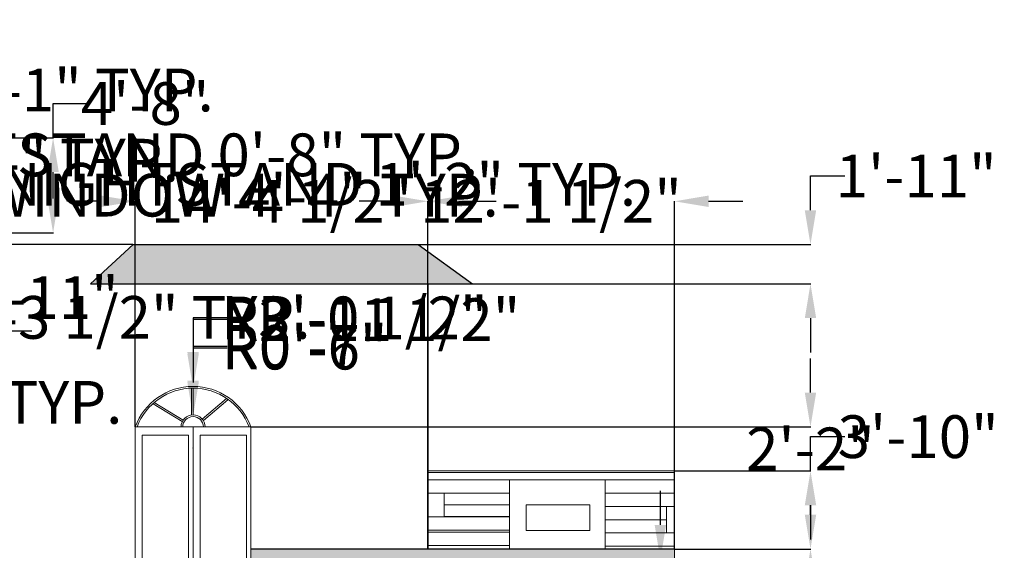
# Model space of a CAD drawing. Units: inches. Extents: x 28 to 3832, y 2 to 1709.
# Tile 6 of 7: x 2956 to 3536, y 1338 to 1651. Entities that reach past the tile are written whole.
import ezdxf

# ---------------------------------------------------------------- set-up
doc = ezdxf.new("R2010")
doc.units = ezdxf.units.IN
doc.header["$MEASUREMENT"] = 0
for name, color, linetype, lineweight in [('A-ANNO-DIMS', 2, 'Continuous', 18), ('A-ELEV', 7, 'Continuous', 30), ('A-ELEV-DETL', 7, 'Continuous', 18), ('A-ELEV-OPEN', 4, 'Continuous', 18), ('A-ELEV-ROOF', 7, 'Continuous', 25)]:
    doc.layers.add(name, color=color, linetype=linetype, lineweight=lineweight)
doc.layers.add('A-ELEV-PATT', color=252, linetype='Continuous', lineweight=9, true_color=0x939598)
doc.layers.add('A-ROOF-PATT', color=30, linetype='Continuous', lineweight=9, true_color=0xf8991e)
doc.styles.get("Standard").update_dxf_attribs({"font": 'arial.ttf'})
doc.dimstyles.get("Standard").update_dxf_attribs({"dimtxt": 25.18, "dimasz": 20.18, "dimexe": 0.18, "dimexo": 0.0625, "dimgap": 0.09, "dimtad": 0, "dimtih": 1, "dimtoh": 1, "dimdec": 0, "dimzin": 0, "dimdsep": 46, "dimlunit": 3, "dimtxsty": 'Standard', "dimcen": 0.09, "dimadec": 0, "dimazin": 0, "dimtfac": 1, "dimtdec": 0, "dimtofl": 0, "dimtmove": 0, "dimatfit": 3, "dimfxl": 1, "dimtolj": 1, "dimtzin": 0, "dimarcsym": 0})

# ---------------------------------------------------------------- blocks, each defined once
blk = doc.blocks.new('*D23')
at = {"layer": 'A-ANNO-DIMS', "color": 0, "lineweight": -2, "transparency": 16777216}
for p, q in [((2540.14, 1405.47), (2540.14, 1425.65)), ((2540.14, 1425.65), (2560.32, 1425.65)), ((2548.79, 1405.47), (2539.96, 1405.47)), ((2540.14, 1367.62), (2540.14, 1385.29)), ((2548.79, 1347.44), (2539.96, 1347.44))]:
    blk.add_line(p, q, dxfattribs=at)
at = {"layer": 'A-ANNO-DIMS', "color": 0, "transparency": 16777216}
for points in [[(2536.78, 1385.29), (2543.51, 1385.29), (2540.14, 1405.47)], [(2536.78, 1367.62), (2543.51, 1367.62), (2540.14, 1347.44)]]:
    blk.add_solid(points, dxfattribs=at)
at = {"layer": 'Defpoints', "color": 0, "transparency": 16777216}
for p in [(2540.14, 1405.47), (2548.85, 1405.47), (2548.85, 1347.44)]:
    blk.add_point(p, dxfattribs=at)
at = {"layer": 'A-ANNO-DIMS', "color": 0, "transparency": 16777216, "insert": (2795, 1425.65), "char_height": 25.18, "attachment_point": 5}
blk.add_mtext('\\A1;WINDOW SHADE 4\'-10" TYP.', dxfattribs=at)
blk = doc.blocks.new('*D25')
at = {"layer": 'A-ANNO-DIMS', "color": 0, "lineweight": -2, "transparency": 16777216}
for p, q in [((2905.84, 1527.52), (2905.84, 1547.7)), ((2905.84, 1547.7), (2926.02, 1547.7)), ((2913.58, 1527.52), (2905.66, 1527.52)), ((2905.84, 1495.7), (2905.84, 1507.34)), ((2913.58, 1475.52), (2905.66, 1475.52))]:
    blk.add_line(p, q, dxfattribs=at)
at = {"layer": 'A-ANNO-DIMS', "color": 0, "transparency": 16777216}
for points in [[(2902.48, 1507.34), (2909.2, 1507.34), (2905.84, 1527.52)], [(2902.48, 1495.7), (2909.2, 1495.7), (2905.84, 1475.52)]]:
    blk.add_solid(points, dxfattribs=at)
at = {"layer": 'Defpoints', "color": 0, "transparency": 16777216}
for p in [(2905.84, 1527.52), (2913.64, 1527.52), (2913.64, 1475.52)]:
    blk.add_point(p, dxfattribs=at)
at = {"layer": 'A-ANNO-DIMS', "color": 0, "transparency": 16777216, "insert": (3085.42, 1547.7), "char_height": 25.18, "attachment_point": 5}
blk.add_mtext('\\A1;WINDOW 4\'-4" TYP.', dxfattribs=at)
blk = doc.blocks.new('*D26')
at = {"layer": 'A-ANNO-DIMS', "color": 0, "lineweight": -2, "transparency": 16777216}
for p, q in [((2913.64, 1475.46), (2913.64, 1467.54)), ((2922.64, 1475.46), (2922.64, 1467.54)), ((2893.46, 1467.72), (2873.28, 1467.72)), ((2942.82, 1467.72), (2963, 1467.72))]:
    blk.add_line(p, q, dxfattribs=at)
at = {"layer": 'A-ANNO-DIMS', "color": 0, "transparency": 16777216}
for points in [[(2893.46, 1471.09), (2893.46, 1464.36), (2913.64, 1467.72)], [(2942.82, 1471.09), (2942.82, 1464.36), (2922.64, 1467.72)]]:
    blk.add_solid(points, dxfattribs=at)
at = {"layer": 'Defpoints', "color": 0, "transparency": 16777216}
for p in [(2913.64, 1475.52), (2922.64, 1475.52), (2913.64, 1467.72)]:
    blk.add_point(p, dxfattribs=at)
at = {"layer": 'A-ANNO-DIMS', "color": 0, "transparency": 16777216, "insert": (2796.45, 1467.72), "char_height": 25.18, "attachment_point": 5}
blk.add_mtext('\\A1;0\'-9" TYP.', dxfattribs=at)
blk = doc.blocks.new('*D31')
at = {"layer": 'A-ANNO-DIMS', "color": 0, "lineweight": -2, "transparency": 16777216}
for p, q in [((2653.18, 1475.69), (2633, 1475.69)), ((2673.36, 1469.86), (2673.36, 1475.87)), ((2712.64, 1469.86), (2712.64, 1475.87)), ((2732.82, 1475.69), (2753, 1475.69))]:
    blk.add_line(p, q, dxfattribs=at)
at = {"layer": 'A-ANNO-DIMS', "color": 0, "transparency": 16777216}
for points in [[(2653.18, 1479.05), (2653.18, 1472.33), (2673.36, 1475.69)], [(2732.82, 1479.05), (2732.82, 1472.33), (2712.64, 1475.69)]]:
    blk.add_solid(points, dxfattribs=at)
at = {"layer": 'Defpoints', "color": 0, "transparency": 16777216}
for p in [(2712.64, 1475.69), (2673.36, 1469.8), (2712.64, 1469.8)]:
    blk.add_point(p, dxfattribs=at)
at = {"layer": 'A-ANNO-DIMS', "color": 0, "transparency": 16777216, "insert": (2943.56, 1475.69), "char_height": 25.18, "attachment_point": 5}
blk.add_mtext('\\A1;DOOR D1 3\'-3 1/2" TYP.', dxfattribs=at)
blk = doc.blocks.new('*D35')
at = {"layer": 'A-ANNO-DIMS', "color": 0, "lineweight": -2, "transparency": 16777216}
for p, q in [((2708.46, 1568.32), (2688.28, 1568.32)), ((2728.64, 1572.46), (2728.64, 1568.14)), ((2756.64, 1572.46), (2756.64, 1568.14)), ((2776.82, 1568.32), (2797, 1568.32))]:
    blk.add_line(p, q, dxfattribs=at)
at = {"layer": 'A-ANNO-DIMS', "color": 0, "transparency": 16777216}
for points in [[(2708.46, 1571.69), (2708.46, 1564.96), (2728.64, 1568.32)], [(2776.82, 1571.69), (2776.82, 1564.96), (2756.64, 1568.32)]]:
    blk.add_solid(points, dxfattribs=at)
at = {"layer": 'Defpoints', "color": 0, "transparency": 16777216}
for p in [(2728.64, 1572.52), (2756.64, 1572.52), (2756.64, 1568.32)]:
    blk.add_point(p, dxfattribs=at)
at = {"layer": 'A-ANNO-DIMS', "color": 0, "transparency": 16777216, "insert": (2926.28, 1568.32), "char_height": 25.18, "attachment_point": 5}
blk.add_mtext('\\A1;VENT 2\'-4" TYP.', dxfattribs=at)
blk = doc.blocks.new('*D39')
at = {"layer": 'A-ANNO-DIMS', "color": 0, "lineweight": -2, "transparency": 16777216}
for p, q in [((2653.75, 1571.46), (2633.57, 1571.46)), ((2673.93, 1570.3), (2673.93, 1571.64)), ((2682.13, 1570.3), (2682.13, 1571.64)), ((2702.31, 1571.46), (2722.49, 1571.46))]:
    blk.add_line(p, q, dxfattribs=at)
at = {"layer": 'A-ANNO-DIMS', "color": 0, "transparency": 16777216}
for points in [[(2653.75, 1574.83), (2653.75, 1568.1), (2673.93, 1571.46)], [(2702.31, 1574.83), (2702.31, 1568.1), (2682.13, 1571.46)]]:
    blk.add_solid(points, dxfattribs=at)
at = {"layer": 'Defpoints', "color": 0, "transparency": 16777216}
for p in [(2673.93, 1570.23), (2682.13, 1571.46), (2682.13, 1570.23)]:
    blk.add_point(p, dxfattribs=at)
at = {"layer": 'A-ANNO-DIMS', "color": 0, "transparency": 16777216, "insert": (2981.04, 1571.46), "char_height": 25.18, "attachment_point": 5}
blk.add_mtext('\\A1;SMALL NIGHTSTAND 0\'-8" TYP.', dxfattribs=at)
blk = doc.blocks.new('*D41')
at = {"layer": 'A-ANNO-DIMS', "color": 0, "lineweight": -2, "transparency": 16777216}
for p, q in [((2881.52, 1556.14), (2881.52, 1553.93)), ((2895.49, 1556.14), (2895.49, 1553.93)), ((2861.34, 1554.11), (2841.16, 1554.11)), ((2915.67, 1554.11), (2935.85, 1554.11))]:
    blk.add_line(p, q, dxfattribs=at)
at = {"layer": 'A-ANNO-DIMS', "color": 0, "transparency": 16777216}
for points in [[(2861.34, 1557.47), (2861.34, 1550.74), (2881.52, 1554.11)], [(2915.67, 1557.47), (2915.67, 1550.74), (2895.49, 1554.11)]]:
    blk.add_solid(points, dxfattribs=at)
at = {"layer": 'Defpoints', "color": 0, "transparency": 16777216}
for p in [(2881.52, 1556.2), (2895.49, 1556.2), (2895.49, 1554.11)]:
    blk.add_point(p, dxfattribs=at)
at = {"layer": 'A-ANNO-DIMS', "color": 0, "transparency": 16777216, "insert": (3131.28, 1554.11), "char_height": 25.18, "attachment_point": 5}
blk.add_mtext('\\A1;NIGHTSTAND 1\'-2" TYP.', dxfattribs=at)
blk = doc.blocks.new('*D42')
at = {"layer": 'A-ANNO-DIMS', "color": 0, "lineweight": -2, "transparency": 16777216}
for p, q in [((2897.58, 1589.46), (2897.58, 1609.64)), ((2897.58, 1609.64), (2917.76, 1609.64)), ((2895.55, 1569.28), (2897.76, 1569.28)), ((2895.55, 1556.2), (2897.76, 1556.2)), ((2897.58, 1536.02), (2897.58, 1515.84))]:
    blk.add_line(p, q, dxfattribs=at)
at = {"layer": 'A-ANNO-DIMS', "color": 0, "transparency": 16777216}
for points in [[(2894.22, 1589.46), (2900.95, 1589.46), (2897.58, 1569.28)], [(2894.22, 1536.02), (2900.95, 1536.02), (2897.58, 1556.2)]]:
    blk.add_solid(points, dxfattribs=at)
at = {"layer": 'Defpoints', "color": 0, "transparency": 16777216}
for p in [(2895.49, 1569.28), (2897.58, 1569.28), (2895.49, 1556.2)]:
    blk.add_point(p, dxfattribs=at)
at = {"layer": 'A-ANNO-DIMS', "color": 0, "transparency": 16777216, "insert": (2993.41, 1609.64), "char_height": 25.18, "attachment_point": 5}
blk.add_mtext('\\A1;1\'-1" TYP.', dxfattribs=at)
blk = doc.blocks.new('*D45')
at = {"layer": 'A-ANNO-DIMS', "color": 0, "lineweight": -2, "transparency": 16777216}
for p, q in [((3166.51, 1302.58), (3166.51, 1280.67)), ((3311.78, 1302.58), (3311.78, 1280.67)), ((3186.69, 1280.85), (3291.6, 1280.85)), ((3311.78, 1280.85), (3331.96, 1280.85))]:
    blk.add_line(p, q, dxfattribs=at)
at = {"layer": 'A-ANNO-DIMS', "color": 0, "transparency": 16777216}
for points in [[(3186.69, 1284.21), (3186.69, 1277.49), (3166.51, 1280.85)], [(3291.6, 1284.21), (3291.6, 1277.49), (3311.78, 1280.85)]]:
    blk.add_solid(points, dxfattribs=at)
at = {"layer": 'Defpoints', "color": 0, "transparency": 16777216}
for p in [(3166.51, 1302.64), (3311.78, 1302.64), (3311.78, 1280.85)]:
    blk.add_point(p, dxfattribs=at)
at = {"layer": 'A-ANNO-DIMS', "color": 0, "transparency": 16777216, "insert": (3590.91, 1280.85), "char_height": 25.18, "attachment_point": 5}
blk.add_mtext('\\A1;ENTRY CANOPY 12\'-1 1/2" TYP.', dxfattribs=at)
blk = doc.blocks.new('*D46')
at = {"layer": 'A-ANNO-DIMS', "color": 0, "lineweight": -2, "transparency": 16777216}
for p, q in [((3333.57, 1353.41), (3333.57, 1373.59)), ((3311.84, 1333.23), (3333.75, 1333.23)), ((3311.84, 1302.64), (3333.75, 1302.64)), ((3333.57, 1282.46), (3333.57, 1262.28))]:
    blk.add_line(p, q, dxfattribs=at)
at = {"layer": 'A-ANNO-DIMS', "color": 0, "transparency": 16777216}
for points in [[(3330.21, 1353.41), (3336.94, 1353.41), (3333.57, 1333.23)], [(3330.21, 1282.46), (3336.94, 1282.46), (3333.57, 1302.64)]]:
    blk.add_solid(points, dxfattribs=at)
at = {"layer": 'Defpoints', "color": 0, "transparency": 16777216}
for p in [(3311.78, 1333.23), (3333.57, 1333.23), (3311.78, 1302.64)]:
    blk.add_point(p, dxfattribs=at)
at = {"layer": 'A-ANNO-DIMS', "color": 0, "transparency": 16777216, "insert": (3333.57, 1317.94), "char_height": 25.18, "attachment_point": 5}
blk.add_mtext('\\A1;2\'-6 1/2" TYP.', dxfattribs=at)
blk = doc.blocks.new('*D51')
at = {"layer": 'A-ANNO-DIMS', "color": 0, "lineweight": -2, "transparency": 16777216}
for p, q in [((2975.53, 1581.52), (2975.53, 1601.7)), ((2975.53, 1601.7), (2995.71, 1601.7)), ((2922.7, 1581.52), (2975.71, 1581.52)), ((2975.53, 1545.7), (2975.53, 1561.34)), ((2922.7, 1525.52), (2975.71, 1525.52))]:
    blk.add_line(p, q, dxfattribs=at)
at = {"layer": 'A-ANNO-DIMS', "color": 0, "transparency": 16777216}
for points in [[(2972.16, 1561.34), (2978.89, 1561.34), (2975.53, 1581.52)], [(2972.16, 1545.7), (2978.89, 1545.7), (2975.53, 1525.52)]]:
    blk.add_solid(points, dxfattribs=at)
at = {"layer": 'Defpoints', "color": 0, "transparency": 16777216}
for p in [(2922.64, 1581.52), (2975.53, 1581.52), (2922.64, 1525.52)]:
    blk.add_point(p, dxfattribs=at)
at = {"layer": 'A-ANNO-DIMS', "color": 0, "transparency": 16777216, "insert": (3029.77, 1601.7), "char_height": 25.18, "attachment_point": 5}
blk.add_mtext('\\A1;4\'-8"', dxfattribs=at)
blk = doc.blocks.new('*D54')
at = {"layer": 'A-ANNO-DIMS', "color": 0, "lineweight": -2, "transparency": 16777216}
for p, q in [((3022.59, 1518.63), (2935.04, 1518.63)), ((2935.22, 1498.45), (2935.22, 1303.17)), ((2935.22, 1081.98), (2935.22, 1277.26)), ((2960.61, 1061.8), (2935.04, 1061.8))]:
    blk.add_line(p, q, dxfattribs=at)
at = {"layer": 'A-ANNO-DIMS', "color": 0, "transparency": 16777216}
for points in [[(2931.86, 1498.45), (2938.58, 1498.45), (2935.22, 1518.63)], [(2931.86, 1081.98), (2938.58, 1081.98), (2935.22, 1061.8)]]:
    blk.add_solid(points, dxfattribs=at)
at = {"layer": 'Defpoints', "color": 0, "transparency": 16777216}
for p in [(2935.22, 1518.63), (3022.65, 1518.63), (2960.67, 1061.8)]:
    blk.add_point(p, dxfattribs=at)
at = {"layer": 'A-ANNO-DIMS', "color": 0, "transparency": 16777216, "insert": (2935.22, 1290.21), "char_height": 25.18, "attachment_point": 5}
blk.add_mtext('\\A1;38\'-1"', dxfattribs=at)
blk = doc.blocks.new('*D55')
at = {"layer": 'A-ANNO-DIMS', "color": 0, "lineweight": -2, "transparency": 16777216}
for p, q in [((3196.43, 1339.29), (3196.43, 1544.26)), ((3341.81, 1339.29), (3341.81, 1544.26)), ((3176.25, 1544.08), (3156.07, 1544.08)), ((3361.99, 1544.08), (3382.17, 1544.08))]:
    blk.add_line(p, q, dxfattribs=at)
at = {"layer": 'A-ANNO-DIMS', "color": 0, "transparency": 16777216}
for points in [[(3176.25, 1547.45), (3176.25, 1540.72), (3196.43, 1544.08)], [(3361.99, 1547.45), (3361.99, 1540.72), (3341.81, 1544.08)]]:
    blk.add_solid(points, dxfattribs=at)
at = {"layer": 'Defpoints', "color": 0, "transparency": 16777216}
for p in [(3341.81, 1544.08), (3196.43, 1339.23), (3341.81, 1339.23)]:
    blk.add_point(p, dxfattribs=at)
at = {"layer": 'A-ANNO-DIMS', "color": 0, "transparency": 16777216, "insert": (3269.12, 1544.08), "char_height": 25.18, "attachment_point": 5}
blk.add_mtext('\\A1;12\'-1 1/2"', dxfattribs=at)
blk = doc.blocks.new('*D56')
at = {"layer": 'A-ANNO-DIMS', "color": 0, "lineweight": -2, "transparency": 16777216}
for p, q in [((3023.98, 1495.5), (3023.98, 1544.26)), ((3196.43, 1495.5), (3196.43, 1544.26)), ((3003.8, 1544.08), (2983.62, 1544.08)), ((3216.61, 1544.08), (3236.79, 1544.08))]:
    blk.add_line(p, q, dxfattribs=at)
at = {"layer": 'A-ANNO-DIMS', "color": 0, "transparency": 16777216}
for points in [[(3003.8, 1547.45), (3003.8, 1540.72), (3023.98, 1544.08)], [(3216.61, 1547.45), (3216.61, 1540.72), (3196.43, 1544.08)]]:
    blk.add_solid(points, dxfattribs=at)
at = {"layer": 'Defpoints', "color": 0, "transparency": 16777216}
for p in [(3196.43, 1544.08), (3023.98, 1495.43), (3196.43, 1495.43)]:
    blk.add_point(p, dxfattribs=at)
at = {"layer": 'A-ANNO-DIMS', "color": 0, "transparency": 16777216, "insert": (3110.2, 1544.08), "char_height": 25.18, "attachment_point": 5}
blk.add_mtext('\\A1;14\'-4 1/2"', dxfattribs=at)
blk = doc.blocks.new('*D61')
at = {"layer": 'A-ANNO-DIMS', "color": 0, "lineweight": -2, "transparency": 16777216}
for p, q in [((3341.88, 1339.23), (3422.25, 1339.23)), ((3422.07, 1319.05), (3422.07, 1289.18)), ((3422.07, 1233.41), (3422.07, 1263.28)), ((3341.88, 1213.23), (3422.25, 1213.23))]:
    blk.add_line(p, q, dxfattribs=at)
at = {"layer": 'A-ANNO-DIMS', "color": 0, "transparency": 16777216}
for points in [[(3418.71, 1319.05), (3425.43, 1319.05), (3422.07, 1339.23)], [(3418.71, 1233.41), (3425.43, 1233.41), (3422.07, 1213.23)]]:
    blk.add_solid(points, dxfattribs=at)
at = {"layer": 'Defpoints', "color": 0, "transparency": 16777216}
for p in [(3341.81, 1339.23), (3422.07, 1339.23), (3341.81, 1213.23)]:
    blk.add_point(p, dxfattribs=at)
at = {"layer": 'A-ANNO-DIMS', "color": 0, "transparency": 16777216, "insert": (3422.07, 1276.23), "char_height": 25.18, "attachment_point": 5}
blk.add_mtext('\\A1;10\'-6"', dxfattribs=at)
blk = doc.blocks.new('*D62')
at = {"layer": 'A-ANNO-DIMS', "color": 0, "lineweight": -2, "transparency": 16777216}
for p, q in [((3422.07, 1385.25), (3422.07, 1405.43)), ((3422.07, 1405.43), (3442.25, 1405.43)), ((3341.88, 1385.25), (3422.25, 1385.25)), ((3422.07, 1359.41), (3422.07, 1365.07)), ((3341.88, 1339.23), (3422.25, 1339.23))]:
    blk.add_line(p, q, dxfattribs=at)
at = {"layer": 'A-ANNO-DIMS', "color": 0, "transparency": 16777216}
for points in [[(3418.71, 1365.07), (3425.43, 1365.07), (3422.07, 1385.25)], [(3418.71, 1359.41), (3425.43, 1359.41), (3422.07, 1339.23)]]:
    blk.add_solid(points, dxfattribs=at)
at = {"layer": 'Defpoints', "color": 0, "transparency": 16777216}
for p in [(3341.81, 1385.25), (3422.07, 1385.25), (3341.81, 1339.23)]:
    blk.add_point(p, dxfattribs=at)
at = {"layer": 'A-ANNO-DIMS', "color": 0, "transparency": 16777216, "insert": (3485.58, 1405.43), "char_height": 25.18, "attachment_point": 5}
blk.add_mtext('\\A1;3\'-10"', dxfattribs=at)
blk = doc.blocks.new('*D63')
at = {"layer": 'A-ANNO-DIMS', "color": 0, "lineweight": -2, "transparency": 16777216}
for p, q in [((3422.07, 1431.36), (3422.07, 1451.54)), ((3092.19, 1411.18), (3422.25, 1411.18)), ((3341.88, 1385.25), (3422.25, 1385.25)), ((3422.07, 1365.07), (3422.07, 1344.89))]:
    blk.add_line(p, q, dxfattribs=at)
at = {"layer": 'A-ANNO-DIMS', "color": 0, "transparency": 16777216}
for points in [[(3418.71, 1431.36), (3425.43, 1431.36), (3422.07, 1411.18)], [(3418.71, 1365.07), (3425.43, 1365.07), (3422.07, 1385.25)]]:
    blk.add_solid(points, dxfattribs=at)
at = {"layer": 'Defpoints', "color": 0, "transparency": 16777216}
for p in [(3092.13, 1411.18), (3422.07, 1411.18), (3341.81, 1385.25)]:
    blk.add_point(p, dxfattribs=at)
at = {"layer": 'A-ANNO-DIMS', "color": 0, "transparency": 16777216, "insert": (3422.07, 1398.21), "char_height": 25.18, "attachment_point": 5}
blk.add_mtext('\\A1;2\'-2"', dxfattribs=at)
blk = doc.blocks.new('*D64')
at = {"layer": 'A-ANNO-DIMS', "color": 0, "lineweight": -2, "transparency": 16777216}
for p, q in [((3422.07, 1538.81), (3422.07, 1558.99)), ((3422.07, 1558.99), (3442.25, 1558.99)), ((3190.79, 1518.63), (3422.25, 1518.63)), ((3222.93, 1495.43), (3422.25, 1495.43)), ((3422.07, 1475.25), (3422.07, 1455.07))]:
    blk.add_line(p, q, dxfattribs=at)
at = {"layer": 'A-ANNO-DIMS', "color": 0, "transparency": 16777216}
for points in [[(3418.71, 1538.81), (3425.43, 1538.81), (3422.07, 1518.63)], [(3418.71, 1475.25), (3425.43, 1475.25), (3422.07, 1495.43)]]:
    blk.add_solid(points, dxfattribs=at)
at = {"layer": 'Defpoints', "color": 0, "transparency": 16777216}
for p in [(3190.73, 1518.63), (3422.07, 1518.63), (3222.87, 1495.43)]:
    blk.add_point(p, dxfattribs=at)
at = {"layer": 'A-ANNO-DIMS', "color": 0, "transparency": 16777216, "insert": (3484.4, 1558.99), "char_height": 25.18, "attachment_point": 5}
blk.add_mtext('\\A1;1\'-11"', dxfattribs=at)
blk = doc.blocks.new('*D69')
at = {"layer": 'A-ANNO-DIMS', "color": 0, "lineweight": -2, "transparency": 16777216}
for p, q in [((2829.79, 1487.38), (2815.4, 1473.22)), ((2849.97, 1487.38), (2829.79, 1487.38)), ((2775.98, 1434.52), (2776.16, 1434.52)), ((2776.07, 1434.43), (2776.07, 1434.61))]:
    blk.add_line(p, q, dxfattribs=at)
at = {"layer": 'A-ANNO-DIMS', "color": 0, "transparency": 16777216}
blk.add_solid([(2813.05, 1475.62), (2817.76, 1470.83), (2801.02, 1459.07)], dxfattribs=at)
at = {"layer": 'Defpoints', "color": 0, "transparency": 16777216}
for p in [(2801.02, 1459.07), (2776.07, 1434.52)]:
    blk.add_point(p, dxfattribs=at)
at = {"layer": 'A-ANNO-DIMS', "color": 0, "transparency": 16777216, "insert": (2932.62, 1487.38), "char_height": 25.18, "attachment_point": 5}
blk.add_mtext('\\A1;2X R2\'-11"', dxfattribs=at)
blk = doc.blocks.new('*D72')
at = {"layer": 'A-ANNO-DIMS', "color": 0, "lineweight": -2, "transparency": 16777216}
for p, q in [((3078.23, 1475.39), (3058.05, 1475.39)), ((3058.05, 1475.39), (3058.05, 1455.21)), ((3057.96, 1398.77), (3058.14, 1398.77)), ((3058.05, 1398.68), (3058.05, 1398.86))]:
    blk.add_line(p, q, dxfattribs=at)
at = {"layer": 'A-ANNO-DIMS', "color": 0, "transparency": 16777216}
blk.add_solid([(3054.69, 1455.21), (3061.42, 1455.21), (3058.05, 1435.03)], dxfattribs=at)
at = {"layer": 'Defpoints', "color": 0, "transparency": 16777216}
for p in [(3058.05, 1435.03), (3058.05, 1398.77)]:
    blk.add_point(p, dxfattribs=at)
at = {"layer": 'A-ANNO-DIMS', "color": 0, "transparency": 16777216, "insert": (3153.18, 1475.39), "char_height": 25.18, "attachment_point": 5}
blk.add_mtext('\\A1;R3\'-0 1/2"', dxfattribs=at)
blk = doc.blocks.new('*D73')
at = {"layer": 'A-ANNO-DIMS', "color": 0, "lineweight": -2, "transparency": 16777216}
for p, q in [((3078.23, 1474.39), (3058.05, 1474.39)), ((3058.05, 1474.39), (3058.05, 1454.21)), ((3057.96, 1398.77), (3058.14, 1398.77)), ((3058.05, 1398.68), (3058.05, 1398.86))]:
    blk.add_line(p, q, dxfattribs=at)
at = {"layer": 'A-ANNO-DIMS', "color": 0, "transparency": 16777216}
blk.add_solid([(3054.69, 1454.21), (3061.42, 1454.21), (3058.05, 1434.03)], dxfattribs=at)
at = {"layer": 'Defpoints', "color": 0, "transparency": 16777216}
for p in [(3058.05, 1434.03), (3058.05, 1398.77)]:
    blk.add_point(p, dxfattribs=at)
at = {"layer": 'A-ANNO-DIMS', "color": 0, "transparency": 16777216, "insert": (3162.96, 1474.39), "char_height": 25.18, "attachment_point": 5}
blk.add_mtext('\\A1;R2\'-11 1/2"', dxfattribs=at)
blk = doc.blocks.new('*D74')
at = {"layer": 'A-ANNO-DIMS', "color": 0, "lineweight": -2, "transparency": 16777216}
for p, q in [((3078.23, 1458.61), (3058.05, 1458.61)), ((3058.05, 1458.61), (3058.05, 1438.43)), ((3057.96, 1411.18), (3058.14, 1411.18)), ((3058.05, 1411.09), (3058.05, 1411.27))]:
    blk.add_line(p, q, dxfattribs=at)
at = {"layer": 'A-ANNO-DIMS', "color": 0, "transparency": 16777216}
blk.add_solid([(3054.69, 1438.43), (3061.42, 1438.43), (3058.05, 1418.25)], dxfattribs=at)
at = {"layer": 'Defpoints', "color": 0, "transparency": 16777216}
for p in [(3058.05, 1418.25), (3058.05, 1411.18)]:
    blk.add_point(p, dxfattribs=at)
at = {"layer": 'A-ANNO-DIMS', "color": 0, "transparency": 16777216, "insert": (3123.84, 1458.61), "char_height": 25.18, "attachment_point": 5}
blk.add_mtext('\\A1;R0\'-7"', dxfattribs=at)
blk = doc.blocks.new('*D75')
at = {"layer": 'A-ANNO-DIMS', "color": 0, "lineweight": -2, "transparency": 16777216}
for p, q in [((3078.23, 1457.61), (3058.05, 1457.61)), ((3058.05, 1457.61), (3058.05, 1437.43)), ((3057.96, 1411.18), (3058.14, 1411.18)), ((3058.05, 1411.09), (3058.05, 1411.27))]:
    blk.add_line(p, q, dxfattribs=at)
at = {"layer": 'A-ANNO-DIMS', "color": 0, "transparency": 16777216}
blk.add_solid([(3054.69, 1437.43), (3061.42, 1437.43), (3058.05, 1417.25)], dxfattribs=at)
at = {"layer": 'Defpoints', "color": 0, "transparency": 16777216}
for p in [(3058.05, 1417.25), (3058.05, 1411.18)]:
    blk.add_point(p, dxfattribs=at)
at = {"layer": 'A-ANNO-DIMS', "color": 0, "transparency": 16777216, "insert": (3123.84, 1457.61), "char_height": 25.18, "attachment_point": 5}
blk.add_mtext('\\A1;R0\'-6"', dxfattribs=at)

msp = doc.modelspace()

# ---------------------------------------------------------------- hatches: boundary and pattern name
at = {"layer": 'A-ELEV-PATT'}
h = msp.add_hatch(color=256, dxfattribs=at)
h.dxf.hatch_style = 1
h.paths.add_polyline_path([(3341.81, 1339.23), (3092.13, 1339.23), (3092.13, 1333.23), (3341.81, 1333.23)])
h.paths.add_polyline_path([(3341.81, 1213.23), (3092.13, 1213.23), (3092.13, 1207.23), (3341.81, 1207.23)])
at = {"layer": 'A-ROOF-PATT'}
h = msp.add_hatch(dxfattribs=at)
h.set_pattern_fill('ANSI38', color=256, scale=8.5)
h.set_pattern_definition([(45, (-138.4383, -52.9559), (-0.75130096, 0.75130096), []), (135, (-138.4383, -52.9559), (-2.25390287, 0.75130096), [2.65625, -1.59375])])
h.paths.add_polyline_path([(3022.65, 1518.63), (2997.52, 1495.43), (3222.87, 1495.43), (3190.73, 1518.63)])

# ---------------------------------------------------------------- linework, layer by layer
at = {"layer": 'A-ELEV'}
for p, q in [((3023.98, 1411.18), (3023.98, 1495.43)), ((3023.98, 1495.43), (3196.43, 1495.43)), ((3196.43, 1495.43), (3196.43, 1339.23)), ((3341.81, 1339.23), (3092.13, 1339.23))]:
    msp.add_line(p, q, dxfattribs=at)
at = {"layer": 'A-ELEV-DETL'}
for p, q in [((3196.43, 1339.23), (3196.43, 1385.25)), ((3196.43, 1385.25), (3341.81, 1385.25)), ((3196.43, 1384.25), (3341.81, 1384.25)), ((3341.81, 1385.25), (3341.81, 1333.23)), ((3244.67, 1379.98), (3196.43, 1379.98)), ((3244.67, 1339.23), (3244.67, 1379.98)), ((3244.67, 1379.98), (3300.98, 1379.98)), ((3300.98, 1379.98), (3300.98, 1339.23)), ((3300.98, 1379.98), (3341.81, 1379.98))]:
    msp.add_line(p, q, dxfattribs=at)
for points in [[(3244.67, 1379.98), (3196.43, 1379.98), (3196.43, 1372.16), (3244.67, 1372.16)], [(3244.67, 1372.16), (3206.14, 1372.16), (3206.14, 1365.28), (3244.67, 1365.28)], [(3244.67, 1365.28), (3206.14, 1365.28), (3206.14, 1358.4), (3244.67, 1358.4)], [(3254.36, 1365.33), (3292.07, 1365.33), (3292.07, 1350.16), (3254.36, 1350.16)], [(3244.67, 1358.23), (3196.43, 1358.23), (3196.43, 1350.41), (3244.67, 1350.41)], [(3244.67, 1349.08), (3196.43, 1349.08), (3196.43, 1341.26), (3244.67, 1341.26)]]:
    msp.add_lwpolyline(points, close=True, dxfattribs=at)
for points in [[(3341.81, 1379.98), (3300.98, 1379.98), (3300.98, 1372.16), (3341.81, 1372.16)], [(3341.81, 1372.16), (3300.98, 1372.16), (3300.98, 1364.35), (3341.81, 1364.35)], [(3300.98, 1356.53), (3337.27, 1356.53), (3337.27, 1364.35), (3300.98, 1364.35)], [(3300.98, 1348.72), (3337.27, 1348.72), (3337.27, 1356.53), (3300.98, 1356.53)], [(3341.81, 1348.72), (3300.98, 1348.72), (3300.98, 1340.9), (3341.81, 1340.9)]]:
    msp.add_lwpolyline(points, dxfattribs=at)
at = {"layer": 'A-ELEV-OPEN'}
for p, q in [((3057.05, 1418.25), (3057.05, 1434.03)), ((3058.05, 1418.25), (3058.05, 1434.03)), ((3051.68, 1414.28), (3034.61, 1424.72)), ((3052.2, 1415.14), (3035.13, 1425.57)), ((3063.47, 1415.72), (3077.86, 1427.95)), ((3064.12, 1414.96), (3078.51, 1427.18)), ((3058.05, 1411.18), (3058.05, 1181.27))]:
    msp.add_line(p, q, dxfattribs=at)
for points in [[(3023.98, 1181.27), (3092.13, 1181.27), (3092.13, 1411.18), (3023.98, 1411.18)], [(3028.11, 1406.28), (3055.43, 1406.28), (3055.43, 1300.77), (3028.11, 1300.77)], [(3062.25, 1406.28), (3089.57, 1406.28), (3089.57, 1300.77), (3062.25, 1300.77)]]:
    msp.add_lwpolyline(points, close=True, dxfattribs=at)
for centre, radius, start, end in [((3058.05, 1398.77), 36.27, 20.01346, 159.98654), ((3058.05, 1398.77), 35.27, 20.60633, 159.39367), ((3058.05, 1411.18), 7.07, 0, 180), ((3058.05, 1411.18), 6.07, 0, 180)]:
    msp.add_arc(centre, radius, start, end, dxfattribs=at)
at = {"layer": 'A-ELEV-ROOF'}
for p, q in [((3022.65, 1518.63), (2997.52, 1495.43)), ((3022.65, 1518.63), (3190.73, 1518.63)), ((3190.73, 1518.63), (3222.87, 1495.43)), ((2997.52, 1495.43), (3222.87, 1495.43))]:
    msp.add_line(p, q, dxfattribs=at)

# ---------------------------------------------------------------- dimensions: what is measured, and where the dimension line sits
at = {"layer": 'A-ANNO-DIMS'}
for base, p1, p2, text, picture, middle in [((2682.13, 1571.46), (2673.93, 1570.23), (2682.13, 1570.23), 'SMALL NIGHTSTAND <> TYP.', '*D39', (2981.04, 1571.46)), ((2756.64, 1568.32), (2728.64, 1572.52), (2756.64, 1572.52), 'VENT <> TYP.', '*D35', (2926.28, 1568.32)), ((2895.49, 1554.11), (2881.52, 1556.2), (2895.49, 1556.2), 'NIGHTSTAND <> TYP.', '*D41', (3131.28, 1554.11)), ((2712.64, 1475.69), (2673.36, 1469.8), (2712.64, 1469.8), 'DOOR D1 <> TYP.', '*D31', (2943.56, 1475.69)), ((3311.78, 1280.85), (3166.51, 1302.64), (3311.78, 1302.64), 'ENTRY CANOPY <> TYP.', '*D45', (3590.91, 1280.85))]:
    dim = msp.add_linear_dim(base=base, p1=p1, p2=p2, text=text, dimstyle='Standard', override={"dimdec": 1, "dimlfac": 1, "dimrnd": 0, "dimzin": 1, "dimdsep": 46, "dimlunit": 4, "dimfrac": 2}, dxfattribs=at)
    dim.commit()
    dim.dimension.update_dxf_attribs({"geometry": picture, "text_midpoint": middle})
for base, p1, p2, angle, text, picture, middle in [((2897.58, 1569.28), (2895.49, 1556.2), (2895.49, 1569.28), 90, '<> TYP.', '*D42', (2993.41, 1609.64)), ((2905.84, 1527.52), (2913.64, 1475.52), (2913.64, 1527.52), 90, 'WINDOW <> TYP.', '*D25', (3085.42, 1547.7)), ((2540.14, 1405.47), (2548.85, 1347.44), (2548.85, 1405.47), 90, 'WINDOW SHADE <> TYP.', '*D23', (2795, 1425.65)), ((2913.64, 1467.72), (2922.64, 1475.52), (2913.64, 1475.52), 180, '<> TYP.', '*D26', (2796.45, 1467.72)), ((3333.57, 1333.23), (3311.78, 1302.64), (3311.78, 1333.23), 90, '<> TYP.', '*D46', (3333.57, 1317.94))]:
    dim = msp.add_linear_dim(base=base, p1=p1, p2=p2, angle=angle, text=text, dimstyle='Standard', override={"dimdec": 1, "dimlfac": 1, "dimrnd": 0, "dimzin": 1, "dimdsep": 46, "dimlunit": 4, "dimfrac": 2}, dxfattribs=at)
    dim.commit()
    dim.dimension.update_dxf_attribs({"geometry": picture, "text_midpoint": middle})
for base, p1, p2, picture, middle in [((2975.53, 1581.52), (2922.64, 1525.52), (2922.64, 1581.52), '*D51', (3029.77, 1601.7)), ((3422.07, 1518.63), (3222.87, 1495.43), (3190.73, 1518.63), '*D64', (3484.4, 1558.99)), ((2935.22, 1518.63), (2960.67, 1061.8), (3022.65, 1518.63), '*D54', (2935.22, 1290.21)), ((3422.07, 1411.18), (3341.81, 1385.25), (3092.13, 1411.18), '*D63', (3422.07, 1398.21)), ((3422.07, 1385.25), (3341.81, 1339.23), (3341.81, 1385.25), '*D62', (3485.58, 1405.43)), ((3422.07, 1339.23), (3341.81, 1213.23), (3341.81, 1339.23), '*D61', (3422.07, 1276.23))]:
    dim = msp.add_linear_dim(base=base, p1=p1, p2=p2, angle=90, dimstyle='Standard', override={"dimdec": 1, "dimlfac": 1, "dimrnd": 0, "dimzin": 1, "dimdsep": 46, "dimlunit": 4, "dimfrac": 2}, dxfattribs=at)
    dim.commit()
    dim.dimension.update_dxf_attribs({"geometry": picture, "text_midpoint": middle})
for base, p1, p2, picture, middle in [((3196.4267, 1544.0828), (3023.9766, 1495.4346), (3196.4267, 1495.4346), '*D56', (3110.2016, 1544.0828)), ((3341.81, 1544.08), (3196.43, 1339.23), (3341.81, 1339.23), '*D55', (3269.12, 1544.08))]:
    dim = msp.add_linear_dim(base=base, p1=p1, p2=p2, dimstyle='Standard', override={"dimdec": 1, "dimlfac": 1, "dimrnd": 0, "dimzin": 1, "dimdsep": 46, "dimlunit": 4, "dimfrac": 2}, dxfattribs=at)
    dim.commit()
    dim.dimension.update_dxf_attribs({"geometry": picture, "text_midpoint": middle})
dim = msp.add_radius_dim(center=(2776.07, 1434.52), mpoint=(2801.02, 1459.07), text='2X <>', dimstyle='Standard', override={"dimdec": 1, "dimlfac": 1, "dimrnd": 0, "dimzin": 1, "dimdsep": 46, "dimlunit": 4, "dimfrac": 2}, dxfattribs=at)
dim.commit()
dim.dimension.update_dxf_attribs({"geometry": '*D69', "text_midpoint": (2932.62, 1487.38)})
for center, mpoint, picture, middle in [((3058.05, 1398.77), (3058.05, 1435.03), '*D72', (3153.18, 1475.39)), ((3058.05, 1398.77), (3058.05, 1434.03), '*D73', (3162.96, 1474.39)), ((3058.05, 1411.18), (3058.05, 1418.25), '*D74', (3123.84, 1458.61)), ((3058.05, 1411.18), (3058.05, 1417.25), '*D75', (3123.84, 1457.61))]:
    dim = msp.add_radius_dim(center=center, mpoint=mpoint, dimstyle='Standard', override={"dimdec": 1, "dimlfac": 1, "dimrnd": 0, "dimzin": 1, "dimdsep": 46, "dimlunit": 4, "dimfrac": 2}, dxfattribs=at)
    dim.commit()
    dim.dimension.update_dxf_attribs({"geometry": picture, "text_midpoint": middle})

doc.saveas('drawing.dxf')
